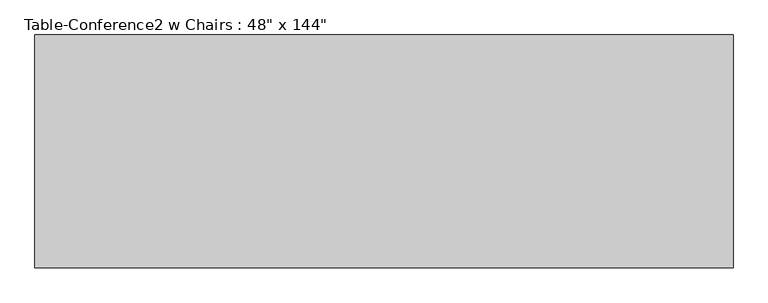
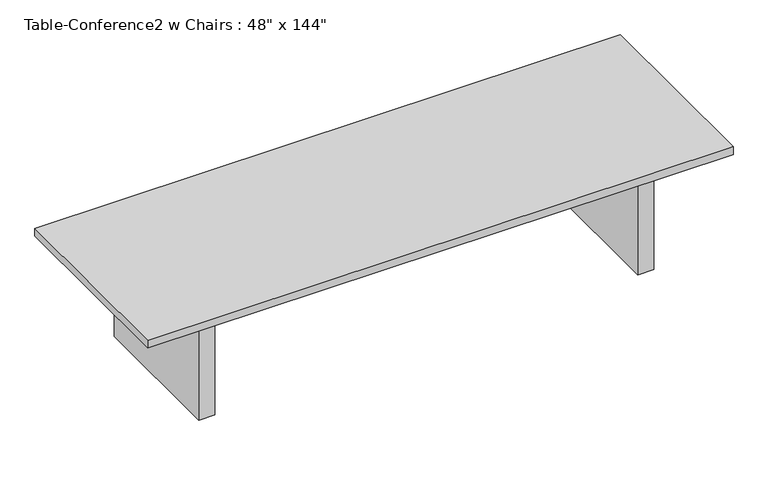
"""IFC4 building model written with IfcOpenShell, lengths in millimetres: furniture geometry."""

from ifc_helpers import new_model, si_unit, frame, origin, origin_with_axes, place, context, project, spatial, polyline, outline, extrude, source, transform, mapped, element, save


def furniture_00fa8475(model_context):
    return source(origin(), model_context, "Body", "SweptSolid", [
        extrude(outline(polyline([(1828.8, -609.6), (-1828.8, -609.6), (-1828.8, 609.6), (1828.8, 609.6), (1828.8, -609.6)])), frame((0.0, 0.0, 711.2), z_axis=(0.0, 0.0, 1.0), x_axis=(1.0, 0.0, 0.0)), (0.0, 0.0, 1.0), 50.8),
        extrude(outline(polyline([(-1320.8, -457.2), (-1422.4, -457.2), (-1422.4, 457.2), (-1320.8, 457.2), (-1320.8, -457.2)])), origin_with_axes(), (0.0, 0.0, 1.0), 711.2),
        extrude(outline(polyline([(1422.4, -457.2), (1320.8, -457.2), (1320.8, 457.2), (1422.4, 457.2), (1422.4, -457.2)])), origin_with_axes(), (0.0, 0.0, 1.0), 711.2),
        extrude(outline(polyline([(1320.8, 457.2), (1320.8, 419.1), (-1320.8, 419.1), (-1320.8, 457.2), (1320.8, 457.2)])), frame((0.0, 0.0, 609.6), z_axis=(0.0, 0.0, 1.0), x_axis=(1.0, 0.0, 0.0)), (0.0, 0.0, 1.0), 101.6),
        extrude(outline(polyline([(1320.8, -457.2), (-1320.8, -457.2), (-1320.8, -419.1), (1320.8, -419.1), (1320.8, -457.2)])), frame((0.0, 0.0, 609.6), z_axis=(0.0, 0.0, 1.0), x_axis=(1.0, 0.0, 0.0)), (0.0, 0.0, 1.0), 101.6),
    ])


if __name__ == "__main__":
    model = new_model("IFC4")
    model_context = context("Model", 3, world=origin())
    ifc_project = project(units=[si_unit("LENGTHUNIT", "METRE", prefix="MILLI")], contexts=[model_context])
    site = spatial("IfcSite", under=ifc_project)
    building = spatial("IfcBuilding", under=site)
    placement = place(None, origin())
    furniture_shape = furniture_00fa8475(model_context)
    element("IfcFurniture", 1, ObjectType="Table-Conference2 w Chairs : 48\" x 144\"", at=placement, inside=building, context=model_context, shape_type="MappedRepresentation", body=[
        mapped(furniture_shape, transform((0.0, 0.0, 0.0), x_axis=(1.0, 0.0, 0.0), y_axis=(0.0, 1.0, 0.0), z_axis=(0.0, 0.0, 1.0))),
    ])
    save(model, "model.ifc")

# Revit data of these elements
# Type "Table-Conference2 w Chairs : 48\" x 144\""
#   Assembly Code = "E2020200"
#   Description = "Seating 12-14"
#   Height = 2' - 6"
#   Length = 12' - 0"
#   Width = 4' - 0"
#   Number Of Chairs One Side = 5
#   Number Of Chairs = 12
#   Material = Wood - Cherry
#   Default Elevation = 0
# Element 1 (IfcFurniture, "Table-Conference2 w Chairs : 48\" x 144\"")
#   Materials on its faces: "Wood - Cherry"
# Materials
#   "Wood - Cherry": colour RGB 151 75 0, transparency 0
